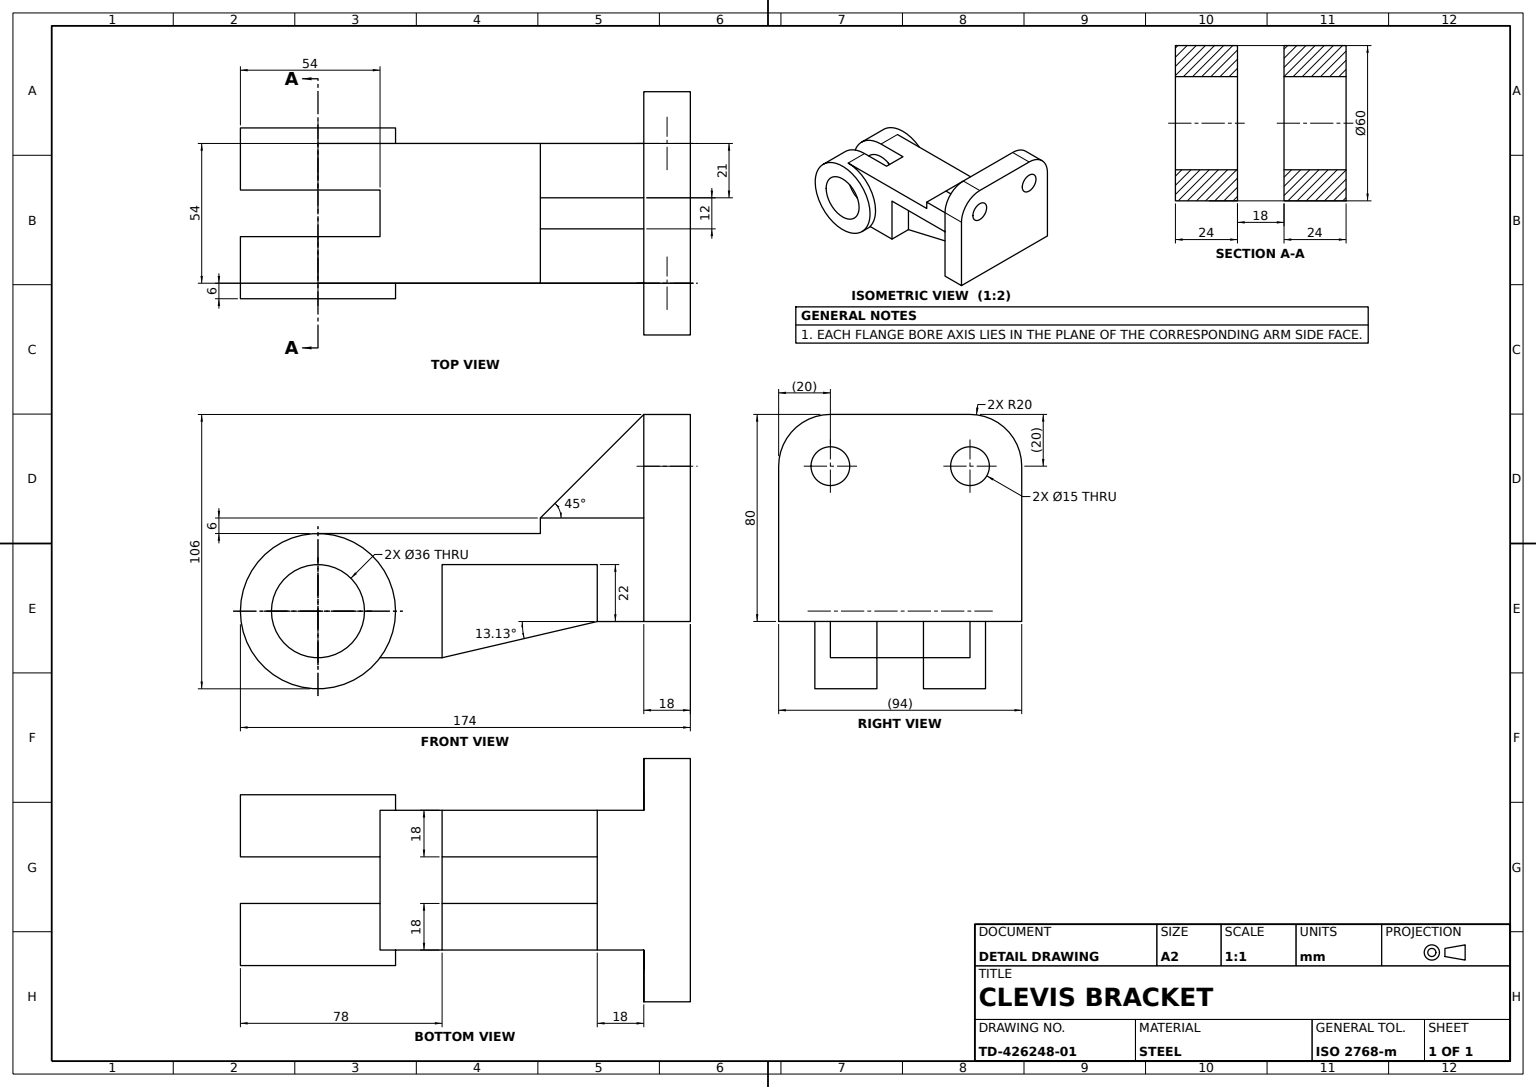
from build123d import *

# Parameters (mm, degrees)
CLEVIS_LUG_A_SKETCH_R       = 30
CLEVIS_LUG_A_SKETCH_R_2     = 18
CLEVIS_LUG_A_60X_36_DEPTH   = 24
CLEVIS_LUG_B_SKETCH_R       = 30
CLEVIS_LUG_B_SKETCH_R_2     = 18
CLEVIS_LUG_B_60X_36_DEPTH   = 24
ARM_START                   = -18
ARM_WEB_DEPTH               = 18
LUG_START                   = -18
LUG_BRIDGE_DEPTH            = 18
ARM_TOP_PLATE_SKETCH_W      = 54
ARM_TOP_PLATE_SKETCH_H      = 40
ARM_TOP_PLATE_6MM_DEPTH     = 6
ARM_SPINE_SKETCH_R          = 4
ARM_SPINE_54MM_DEPTH        = 54
ARM_BODY_SKETCH_W           = 18
ARM_BODY_SKETCH_H           = 22
ARM_BODY_80MM_DEPTH         = 80
ARM_SIDE_WEB_54MM_DEPTH     = 54
ARM_SLOT_SKETCH_W           = 24
ARM_SLOT_SKETCH_H           = 6
ARM_SLOT_CUT_DEPTH          = 27
ARM_RIB_18MM_REACH          = 137.133
ARM_RIB_SKETCH_WALL_W       = 333.878222312
ARM_RIB_SKETCH_WALL_H       = 18
MOUNTING_FLANGE_SKETCH_R    = 7.5
MOUNTING_FLANGE_DEPTH       = 18
FLANGE_GUSSET_12MM_REACH    = 171.473
FLANGE_GUSSET_SKETCH_WALL_W = 397.51396583
FLANGE_GUSSET_SKETCH_WALL_H = 12


with BuildPart() as part:
    # Clevis Lug A Sketch → Clevis Lug A Ø60xØ36 (new body)
    with BuildSketch(Plane(origin=(0, 0, 0), x_dir=(0, 0, -1), z_dir=(1, 0, 0))):
        Circle(CLEVIS_LUG_A_SKETCH_R)
        Circle(CLEVIS_LUG_A_SKETCH_R_2, mode=Mode.SUBTRACT)
    extrude(amount=CLEVIS_LUG_A_60X_36_DEPTH)

    # Arm Web Sketch → Arm Web (add)
    with BuildSketch(Plane(origin=(18, 0, 0), x_dir=(0, 0, -1), z_dir=(1, 0, 0)).offset(ARM_START)):
        with BuildLine():
            Line((0, 30), (48, 30))
            Line((48, 30), (126, 30))
            Line((126, 30), (126, -4))
            Line((126, -4), (108, -4))
            Line((108, -4), (108, 18))
            Line((108, 18), (48, 18))
            Line((48, 18), (48, -4))
            Line((48, -4), (17.549928775, -4))
            ThreePointArc((17.549928775, -4), (14.071247279, 11.22497216), (0, 18))
            Line((0, 18), (0, 30))
        make_face()
    extrude(amount=ARM_WEB_DEPTH)



with BuildPart() as body_2:
    # Clevis Lug B Sketch → Clevis Lug B Ø60xØ36 (new body)
    with BuildSketch(Plane(origin=(-18, 0, 0), x_dir=(0, 0, -1), z_dir=(1, 0, 0))):
        Circle(CLEVIS_LUG_B_SKETCH_R)
        Circle(CLEVIS_LUG_B_SKETCH_R_2, mode=Mode.SUBTRACT)
    extrude(amount=-CLEVIS_LUG_B_60X_36_DEPTH)

    # Lug Bridge Sketch → Lug Bridge (add)
    with BuildSketch(Plane(origin=(-18, 0, 0), x_dir=(0, 0, -1), z_dir=(1, 0, 0)).offset(LUG_START)):
        with BuildLine():
            Line((0, 30), (126, 30))
            Line((126, 30), (126, -4))
            Line((126, -4), (108, -4))
            Line((108, -4), (108, 18))
            Line((108, 18), (48, 18))
            Line((48, 18), (48, -4))
            Line((48, -4), (17.549928775, -4))
            ThreePointArc((17.549928775, -4), (14.071247279, 11.22497216), (0, 18))
            Line((0, 18), (0, 30))
        make_face()
    extrude(amount=LUG_BRIDGE_DEPTH)


with BuildPart() as part_1:
    add(part.part)

    add(body_2.part)  # Arm Top Plate 6mm merges body 2
    # Arm Top Plate Sketch → Arm Top Plate 6mm (add)
    with BuildSketch(Plane(origin=(0, 30, 0), x_dir=(1, 0, 0), z_dir=(0, 1, 0))):
        with Locations((-9, 106)):
            Rectangle(ARM_TOP_PLATE_SKETCH_W, ARM_TOP_PLATE_SKETCH_H)
    extrude(amount=ARM_TOP_PLATE_6MM_DEPTH)

    # Arm Spine Sketch → Arm Spine 54mm (add)
    with BuildSketch(Plane(origin=(18, 0, 0), x_dir=(0, 0, -1), z_dir=(1, 0, 0))):
        with BuildLine():
            ThreePointArc((24, 18), (29.030770743, 7.564016794), (29.732137495, -4))
            Line((29.732137495, -4), (48, -4))
            Line((48, -4), (48, 18))
            Line((48, 18), (108, 18))
            Line((108, 18), (126, 18))
            Line((126, 18), (126, 30))
            Line((126, 30), (86, 30))
            Line((86, 30), (24, 30))
            Line((24, 30), (24, 18))
        make_face()
        with BuildLine():
            Line((24, 18), (24, -4))
            Line((24, -4), (29.732137495, -4))
            ThreePointArc((29.732137495, -4), (29.030770743, 7.564016794), (24, 18))
        make_face()
        Circle(ARM_SPINE_SKETCH_R)
    extrude(amount=-ARM_SPINE_54MM_DEPTH)


with BuildPart() as arm_spine_54mm_kept_piece:
    # of the separate pieces the step leaves, the one the design keeps (arm_spine_54mm_pieces_kept)
    add(part_1.part.solids().sort_by_distance((-36, 36, -126))[0])

    # Arm Body Sketch → Arm Body 80mm (add)
    with BuildSketch(Plane(origin=(0, 0, -126), x_dir=(-1, 0, 0), z_dir=(0, 0, -1))):
        with Locations((9, 7)):
            Rectangle(ARM_BODY_SKETCH_W, ARM_BODY_SKETCH_H)
    extrude(amount=-ARM_BODY_80MM_DEPTH)

    # Arm Side Web Sketch → Arm Side Web 54mm (add)
    with BuildSketch(Plane(origin=(18, 0, 0), x_dir=(0, 0, -1), z_dir=(1, 0, 0))):
        Polygon((48, -4), (48, -24), (24, -24), (24, 6), (48, 6), align=None)
    extrude(amount=-ARM_SIDE_WEB_54MM_DEPTH)

    # Arm Slot Sketch → Arm Slot Cut (cut, symmetric)
    with BuildSketch(Plane(origin=(-9, 0, 0), x_dir=(0, 0, -1), z_dir=(1, 0, 0))):
        with Locations((36, -21)):
            Rectangle(ARM_SLOT_SKETCH_W, ARM_SLOT_SKETCH_H)
    extrude(amount=ARM_SLOT_CUT_DEPTH, both=True, mode=Mode.SUBTRACT)

    # Arm Rib Sketch wall → Arm Rib 18mm (add, up to next)
    with BuildSketch(Plane(origin=(-9, -11, -78), x_dir=(0, 0.227229615606, -0.973841209742), z_dir=(0, 0.973841209742, 0.227229615606)), mode=Mode.PRIVATE) as arm_rib_18mm_sk1:
        Rectangle(ARM_RIB_SKETCH_WALL_W, ARM_RIB_SKETCH_WALL_H)
    arm_rib_18mm_tool1 = extrude(arm_rib_18mm_sk1.sketch, amount=ARM_RIB_18MM_REACH, mode=Mode.PRIVATE) - arm_spine_54mm_kept_piece.part
    add(arm_rib_18mm_tool1.solids().sort_by_distance((-9, -11, -78))[0])

    # Mounting Flange Sketch → Mounting Flange (add)
    with BuildSketch(Plane(origin=(0, 0, -126), x_dir=(-1, 0, 0), z_dir=(0, 0, -1))):
        with BuildLine():
            Line((-18, 76), (36, 76))
            ThreePointArc((36, 76), (50.142135624, 70.142135624), (56, 56))
            Line((56, 56), (56, -4))
            Line((56, -4), (-38, -4))
            Line((-38, -4), (-38, 56))
            ThreePointArc((-38, 56), (-32.142135624, 70.142135624), (-18, 76))
        make_face()
        with Locations((-18, 56)):
            Circle(MOUNTING_FLANGE_SKETCH_R, mode=Mode.SUBTRACT)
        with Locations((36, 56)):
            Circle(MOUNTING_FLANGE_SKETCH_R, mode=Mode.SUBTRACT)
    extrude(amount=MOUNTING_FLANGE_DEPTH)

    # Flange Gusset Sketch wall → Flange Gusset 12mm (add, up to next)
    with BuildSketch(Plane(origin=(-9, 56, -106), x_dir=(0, 0.707106781187, -0.707106781187), z_dir=(0, 0.707106781187, 0.707106781187)), mode=Mode.PRIVATE) as flange_gusset_12mm_sk1:
        Rectangle(FLANGE_GUSSET_SKETCH_WALL_W, FLANGE_GUSSET_SKETCH_WALL_H)
    flange_gusset_12mm_tool1 = extrude(flange_gusset_12mm_sk1.sketch, amount=-FLANGE_GUSSET_12MM_REACH, mode=Mode.PRIVATE) - arm_spine_54mm_kept_piece.part
    add(flange_gusset_12mm_tool1.solids().sort_by_distance((-9, 56, -106))[0])


solid = arm_spine_54mm_kept_piece.part
